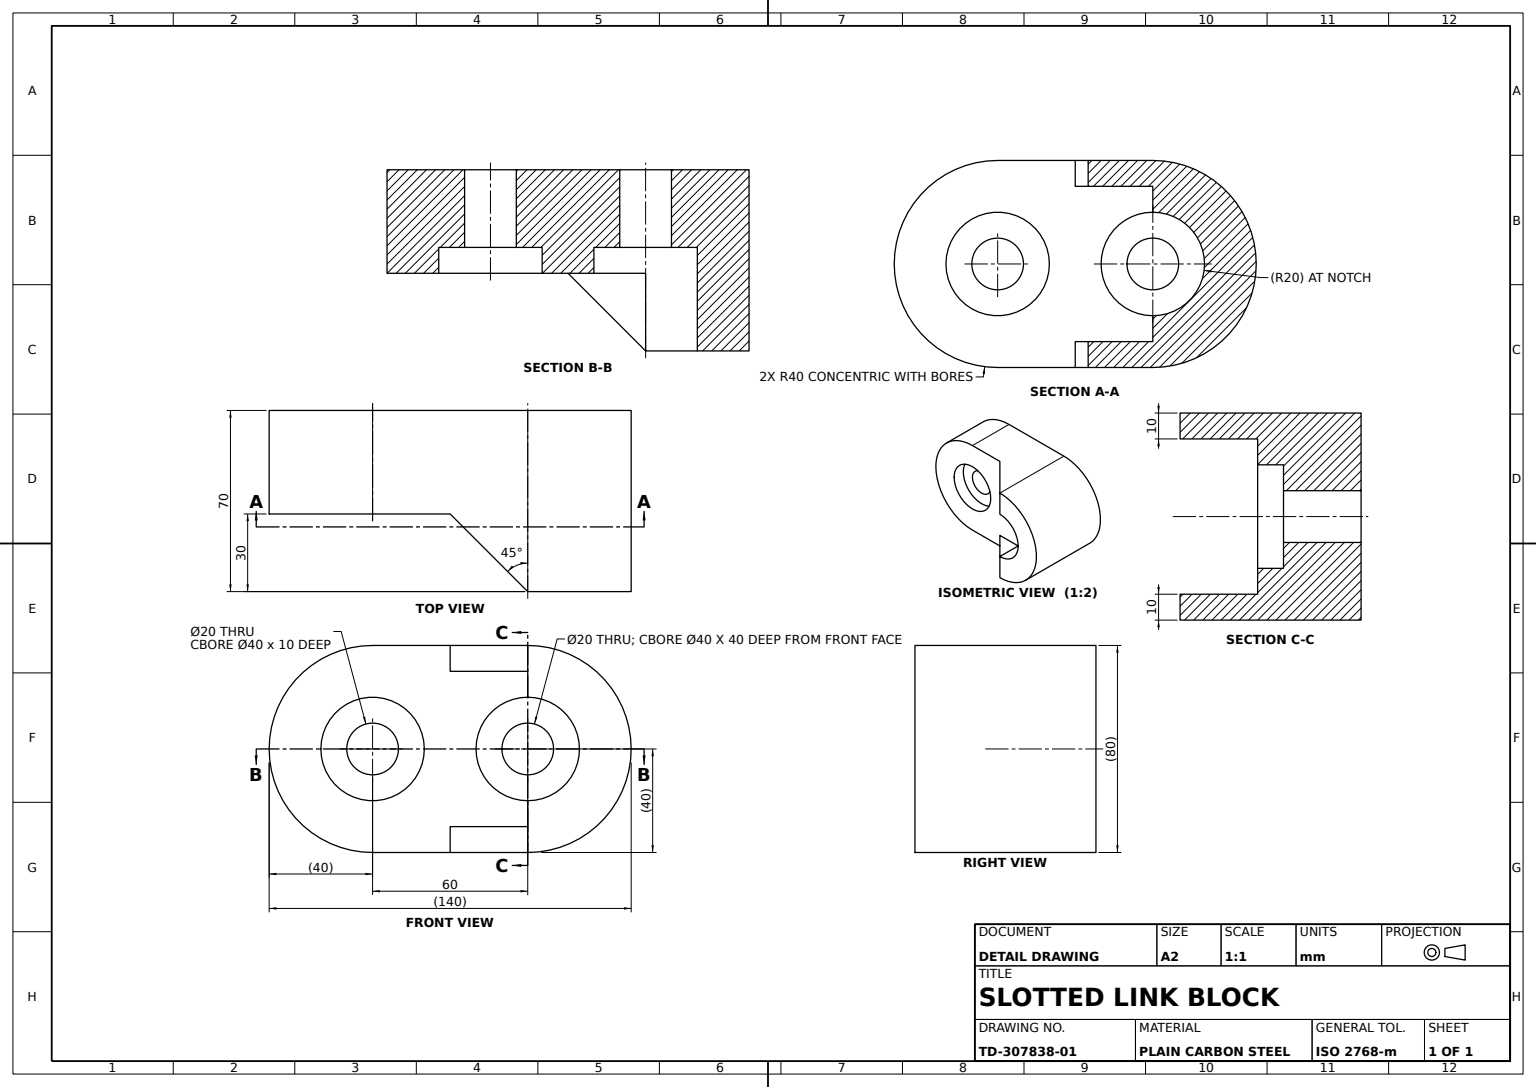
SolidWorks part; units mm, degrees
material "Plain Carbon Steel"
ref_plane "Front Plane" through (0, 0, 0) normal (0, 0, 1) x (1, 0, 0)
ref_plane "Top Plane" through (0, 0, 0) normal (0, 1, 0) x (1, 0, 0)
ref_plane "Right Plane" through (0, 0, 0) normal (1, 0, 0) x (0, 0, -1)
sketch "Base Block Sketch" plane through (0, 0, 0) normal (0, 0, 1) x (1, 0, 0)
  line L1 (0, 40) -> (60, 40)
  line L3 (60, -40) -> (0, -40)
  arc A0 (0, 40) -> (0, -40) centre (0, 0) ccw
  arc A1 (60, -40) -> (60, 40) centre (60, 0) ccw
  dimension "D1" = 80
  dimension "D2" = 80
  dimension "D3" = 40
  dimension "D4" = 60
extrude "Base Block 80x80x40" add sketch "Base Block Sketch" along normal blind 40
sketch "Counterbore 1 Sketch" plane through (0, 0, 40) normal (0, 0, 1) x (1, 0, 0)
  circle A0 centre (0, 0) radius 20
  dimension "D1" = 40
  dimension "D2" = 40
extrude "Counterbore 1 Ø40x10" cut sketch "Counterbore 1 Sketch" against normal blind 10
sketch "Bore 1 Sketch" plane through (0, 0, 30) normal (0, 0, 1) x (1, 0, 0)
  circle A0 centre (0, 0) radius 10
  dimension "D1" = 20
  dimension "D2" = 20
extrude "Bore 1 Ø20" cut sketch "Bore 1 Sketch" against normal blind 30
sketch "Side Boss Sketch" plane through (0, 0, 40) normal (0, 0, 1) x (1, 0, 0)
  line L0 (60, 40) -> (60, -40)
  arc A0 (60, -40) -> (60, 40) centre (60, 0) ccw
  dimension "D1" = 80
extrude "Side Boss" add sketch "Side Boss Sketch" along normal blind 30
sketch "Side Boss Trim Sketch" plane through (0, 0, 70) normal (0, 0, 1) x (1, 0, 0)
  line L0 (60, 40) -> (60, -40) construction
  line L1 (60, 20) -> (60, -20)
  arc A0 (60, -20) -> (60, 20) centre (60, 0) ccw
  dimension "D1" = 40
  dimension "D2" = 20
extrude "Side Boss Trim Cut" cut sketch "Side Boss Trim Sketch" against normal blind 30
sketch "Counterbore 2 Sketch" plane through (0, 0, 40) normal (0, 0, 1) x (1, 0, 0)
  circle A0 centre (60, 0) radius 20
  dimension "D1" = 40
  dimension "D2" = 40
extrude "Counterbore 2 Ø40x10" cut sketch "Counterbore 2 Sketch" against normal blind 10
sketch "Bore 2 Sketch" plane through (0, 0, 30) normal (0, 0, 1) x (1, 0, 0)
  circle A0 centre (60, 0) radius 10
  dimension "D1" = 20
  dimension "D2" = 20
extrude "Bore 2 Ø20" cut sketch "Bore 2 Sketch" against normal blind 30
sketch "Gusset 1 Sketch" plane through (0, -40, 0) normal (0, -1, 0) x (1, 0, 0)
  line L0 (60, 70) -> (60, 40)
  line L1 (60, 40) -> (30, 40)
  line L2 (0, 40) -> (60, 40) construction
  line L3 (30, 40) -> (60, 70)
extrude "Gusset 1" add sketch "Gusset 1 Sketch" against normal blind 10
sketch "Gusset 2 Sketch" plane through (0, 40, 0) normal (0, 1, 0) x (1, 0, 0)
  line L0 (60, -70) -> (60, -40)
  line L1 (60, -40) -> (30, -40)
  line L2 (60, -40) -> (0, -40) construction
  line L3 (30, -40) -> (60, -70)
extrude "Gusset 2" add sketch "Gusset 2 Sketch" against normal blind 10
